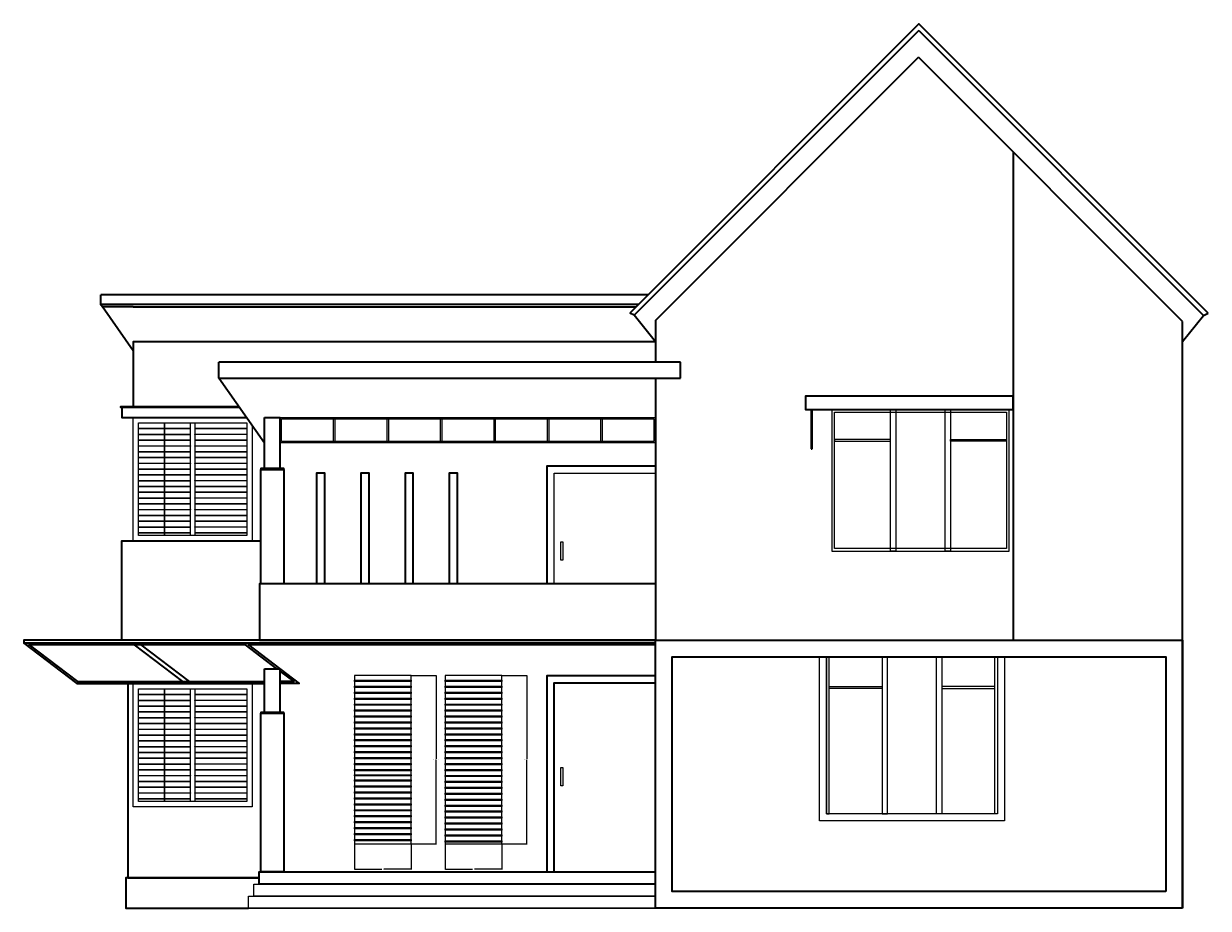
# Model space of a CAD drawing. Units: feet. Extents: x 2613 to 3913, y 950 to 1393.
# Tile 6 of 6: x 3319 to 3913, y 950 to 1393. Entities that reach past the tile are written whole.
import ezdxf

# ---------------------------------------------------------------- set-up
doc = ezdxf.new("R2010")
doc.units = ezdxf.units.FT
for name, color, linetype, lineweight in [('A-ANNO-DIMS', 2, 'Continuous', 18), ('A-DOOR', 3, 'Continuous', 25), ('A-ELEV', 7, 'Continuous', 35), ('A-FLOR-STRS', 7, 'Continuous', 25), ('A-GLAZ', 4, 'Continuous', 25), ('A-ROOF', 1, 'Continuous', 35)]:
    doc.layers.add(name, color=color, linetype=linetype, lineweight=lineweight)
doc.styles.get("Standard").update_dxf_attribs({"font": 'arial.ttf'})
doc.dimstyles.get("Standard").update_dxf_attribs({"dimtxt": 0.18, "dimasz": 0.18, "dimexe": 0.18, "dimexo": 0.0625, "dimgap": 0.09, "dimtad": 0, "dimtih": 1, "dimtoh": 1, "dimdec": 1, "dimzin": 0, "dimdsep": 46, "dimlunit": 3, "dimtxsty": 'Standard', "dimcen": 0.09, "dimadec": 0, "dimazin": 0, "dimtfac": 1, "dimtdec": 1, "dimtofl": 0, "dimtmove": 0, "dimatfit": 3, "dimfxl": 1, "dimtolj": 1, "dimtzin": 0, "dimarcsym": 0})

# ---------------------------------------------------------------- blocks, each defined once
blk = doc.blocks.new('WIN-LOUVRE-SHUTTER-L')
for points in [[(3513.53, 1066.37), (3485.15, 1066.37), (3485.15, 982.04), (3513.53, 982.04)], [(3485.15, 1064.05), (3513.53, 1064.05), (3513.53, 1063.39), (3485.15, 1063.39)], [(3485.15, 1061.07), (3513.53, 1061.07), (3513.53, 1060.41), (3485.15, 1060.41)], [(3485.15, 1058.09), (3513.53, 1058.09), (3513.53, 1057.43), (3485.15, 1057.43)], [(3485.15, 1055.11), (3513.53, 1055.11), (3513.53, 1054.45), (3485.15, 1054.45)], [(3485.15, 1052.13), (3513.53, 1052.13), (3513.53, 1051.47), (3485.15, 1051.47)], [(3485.15, 1049.15), (3513.53, 1049.15), (3513.53, 1048.49), (3485.15, 1048.49)], [(3485.15, 1046.18), (3513.53, 1046.18), (3513.53, 1045.51), (3485.15, 1045.51)], [(3485.15, 1043.2), (3513.53, 1043.2), (3513.53, 1042.53), (3485.15, 1042.53)], [(3485.15, 1040.22), (3513.53, 1040.22), (3513.53, 1039.56), (3485.15, 1039.56)], [(3485.15, 1037.24), (3513.53, 1037.24), (3513.53, 1036.58), (3485.15, 1036.58)], [(3485.15, 1034.26), (3513.53, 1034.26), (3513.53, 1033.6), (3485.15, 1033.6)], [(3485.15, 1031.28), (3513.53, 1031.28), (3513.53, 1030.62), (3485.15, 1030.62)], [(3485.15, 1028.3), (3513.53, 1028.3), (3513.53, 1027.64), (3485.15, 1027.64)], [(3485.15, 1025.32), (3513.53, 1025.32), (3513.53, 1024.66), (3485.15, 1024.66)], [(3485.15, 1022.34), (3513.53, 1022.34), (3513.53, 1021.68), (3485.15, 1021.68)], [(3485.15, 1019.36), (3513.53, 1019.36), (3513.53, 1018.7), (3485.15, 1018.7)], [(3485.15, 1016.71), (3513.53, 1016.71), (3513.53, 1016.05), (3485.15, 1016.05)], [(3485.15, 1014.07), (3513.53, 1014.07), (3513.53, 1013.4), (3485.15, 1013.4)], [(3485.15, 1011.09), (3513.53, 1011.09), (3513.53, 1010.43), (3485.15, 1010.43)], [(3485.15, 1008.11), (3513.53, 1008.11), (3513.53, 1007.45), (3485.15, 1007.45)], [(3485.15, 1005.13), (3513.53, 1005.13), (3513.53, 1004.47), (3485.15, 1004.47)], [(3485.15, 1002.15), (3513.53, 1002.15), (3513.53, 1001.49), (3485.15, 1001.49)], [(3485.15, 999.17), (3513.53, 999.17), (3513.53, 998.51), (3485.15, 998.51)], [(3485.15, 996.19), (3513.53, 996.19), (3513.53, 995.53), (3485.15, 995.53)], [(3485.15, 993.21), (3513.53, 993.21), (3513.53, 992.55), (3485.15, 992.55)], [(3485.15, 990.23), (3513.53, 990.23), (3513.53, 989.57), (3485.15, 989.57)], [(3485.15, 987.25), (3513.53, 987.25), (3513.53, 986.59), (3485.15, 986.59)], [(3485.15, 984.27), (3513.53, 984.27), (3513.53, 983.61), (3485.15, 983.61)]]:
    blk.add_lwpolyline(points, close=True)
blk = doc.blocks.new('WIN-LOUVRE-SHUTTER-R')
for points in [[(3559, 1066.37), (3530.62, 1066.37), (3530.62, 982.04), (3559, 982.04)], [(3530.62, 1064.05), (3559, 1064.05), (3559, 1063.39), (3530.62, 1063.39)], [(3530.62, 1061.07), (3559, 1061.07), (3559, 1060.41), (3530.62, 1060.41)], [(3530.62, 1058.09), (3559, 1058.09), (3559, 1057.43), (3530.62, 1057.43)], [(3530.62, 1055.11), (3559, 1055.11), (3559, 1054.45), (3530.62, 1054.45)], [(3530.62, 1052.13), (3559, 1052.13), (3559, 1051.47), (3530.62, 1051.47)], [(3530.62, 1049.15), (3559, 1049.15), (3559, 1048.49), (3530.62, 1048.49)], [(3530.62, 1046.18), (3559, 1046.18), (3559, 1045.51), (3530.62, 1045.51)], [(3530.62, 1043.2), (3559, 1043.2), (3559, 1042.53), (3530.62, 1042.53)], [(3530.62, 1040.22), (3559, 1040.22), (3559, 1039.56), (3530.62, 1039.56)], [(3530.62, 1037.24), (3559, 1037.24), (3559, 1036.58), (3530.62, 1036.58)], [(3530.62, 1034.26), (3559, 1034.26), (3559, 1033.6), (3530.62, 1033.6)], [(3530.62, 1031.28), (3559, 1031.28), (3559, 1030.62), (3530.62, 1030.62)], [(3530.62, 1028.3), (3559, 1028.3), (3559, 1027.64), (3530.62, 1027.64)], [(3530.62, 1025.32), (3559, 1025.32), (3559, 1024.66), (3530.62, 1024.66)], [(3530.62, 1022.34), (3559, 1022.34), (3559, 1021.68), (3530.62, 1021.68)], [(3530.62, 1019.36), (3559, 1019.36), (3559, 1018.7), (3530.62, 1018.7)], [(3530.62, 1016.38), (3559, 1016.38), (3559, 1015.72), (3530.62, 1015.72)], [(3530.62, 1013.4), (3559, 1013.4), (3559, 1012.74), (3530.62, 1012.74)], [(3530.62, 1010.43), (3559, 1010.43), (3559, 1009.76), (3530.62, 1009.76)], [(3530.62, 1007.45), (3559, 1007.45), (3559, 1006.78), (3530.62, 1006.78)], [(3530.62, 1004.47), (3559, 1004.47), (3559, 1003.81), (3530.62, 1003.81)], [(3530.62, 1001.49), (3559, 1001.49), (3559, 1000.83), (3530.62, 1000.83)], [(3530.62, 998.51), (3559, 998.51), (3559, 997.85), (3530.62, 997.85)], [(3530.62, 995.53), (3559, 995.53), (3559, 994.87), (3530.62, 994.87)], [(3530.62, 992.55), (3559, 992.55), (3559, 991.89), (3530.62, 991.89)], [(3530.62, 989.57), (3559, 989.57), (3559, 988.91), (3530.62, 988.91)], [(3530.62, 986.59), (3559, 986.59), (3559, 985.93), (3530.62, 985.93)], [(3530.62, 983.61), (3559, 983.61), (3559, 982.95), (3530.62, 982.95)]]:
    blk.add_lwpolyline(points, close=True)
blk = doc.blocks.new('*D3')
at = {"layer": 'A-ANNO-DIMS', "color": 0, "lineweight": -2, "transparency": 16777216}
for p, q in [((3513.59, 1066.37), (3526.36, 1066.37)), ((3526.18, 1066.19), (3526.18, 1024.41)), ((3526.18, 982.22), (3526.18, 1023.99)), ((3513.59, 982.04), (3526.36, 982.04))]:
    blk.add_line(p, q, dxfattribs=at)
at = {"layer": 'A-ANNO-DIMS', "color": 0, "transparency": 16777216}
for points in [[(3526.15, 1066.19), (3526.21, 1066.19), (3526.18, 1066.37)], [(3526.15, 982.22), (3526.21, 982.22), (3526.18, 982.04)]]:
    blk.add_solid(points, dxfattribs=at)
at = {"layer": 'Defpoints', "color": 0, "transparency": 16777216}
for p in [(3513.53, 1066.37), (3526.18, 1066.37), (3513.53, 982.04)]:
    blk.add_point(p, dxfattribs=at)
at = {"layer": 'A-ANNO-DIMS', "color": 0, "transparency": 16777216, "insert": (3526.18, 1024.2), "char_height": 0.18, "attachment_point": 5}
blk.add_mtext('\\A1;LOUVRE SHUTTER (L) 84 TYP.', dxfattribs=at)
blk = doc.blocks.new('*D4')
at = {"layer": 'A-ANNO-DIMS', "color": 0, "lineweight": -2, "transparency": 16777216}
for p, q in [((3485.15, 981.97), (3485.15, 969.21)), ((3513.53, 981.97), (3513.53, 969.21)), ((3485.33, 969.39), (3498.81, 969.39)), ((3513.35, 969.39), (3499.87, 969.39))]:
    blk.add_line(p, q, dxfattribs=at)
at = {"layer": 'A-ANNO-DIMS', "color": 0, "transparency": 16777216}
for points in [[(3485.33, 969.42), (3485.33, 969.36), (3485.15, 969.39)], [(3513.35, 969.42), (3513.35, 969.36), (3513.53, 969.39)]]:
    blk.add_solid(points, dxfattribs=at)
at = {"layer": 'Defpoints', "color": 0, "transparency": 16777216}
for p in [(3485.15, 982.04), (3513.53, 982.04), (3513.53, 969.39)]:
    blk.add_point(p, dxfattribs=at)
at = {"layer": 'A-ANNO-DIMS', "color": 0, "transparency": 16777216, "insert": (3499.34, 969.39), "char_height": 0.18, "attachment_point": 5}
blk.add_mtext('\\A1;28 TYP.', dxfattribs=at)
blk = doc.blocks.new('*D5')
at = {"layer": 'A-ANNO-DIMS', "color": 0, "lineweight": -2, "transparency": 16777216}
for p, q in [((3559.06, 1066.37), (3571.83, 1066.37)), ((3571.65, 1066.19), (3571.65, 1024.41)), ((3571.65, 982.22), (3571.65, 1023.99)), ((3559.06, 982.04), (3571.83, 982.04))]:
    blk.add_line(p, q, dxfattribs=at)
at = {"layer": 'A-ANNO-DIMS', "color": 0, "transparency": 16777216}
for points in [[(3571.62, 1066.19), (3571.68, 1066.19), (3571.65, 1066.37)], [(3571.62, 982.22), (3571.68, 982.22), (3571.65, 982.04)]]:
    blk.add_solid(points, dxfattribs=at)
at = {"layer": 'Defpoints', "color": 0, "transparency": 16777216}
for p in [(3559, 1066.37), (3571.65, 1066.37), (3559, 982.04)]:
    blk.add_point(p, dxfattribs=at)
at = {"layer": 'A-ANNO-DIMS', "color": 0, "transparency": 16777216, "insert": (3571.65, 1024.2), "char_height": 0.18, "attachment_point": 5}
blk.add_mtext('\\A1;LOUVRE SHUTTER (R) 84 TYP.', dxfattribs=at)
blk = doc.blocks.new('*D6')
at = {"layer": 'A-ANNO-DIMS', "color": 0, "lineweight": -2, "transparency": 16777216}
for p, q in [((3530.62, 981.97), (3530.62, 969.21)), ((3559, 981.97), (3559, 969.21)), ((3530.8, 969.39), (3544.28, 969.39)), ((3558.82, 969.39), (3545.34, 969.39))]:
    blk.add_line(p, q, dxfattribs=at)
at = {"layer": 'A-ANNO-DIMS', "color": 0, "transparency": 16777216}
for points in [[(3530.8, 969.42), (3530.8, 969.36), (3530.62, 969.39)], [(3558.82, 969.42), (3558.82, 969.36), (3559, 969.39)]]:
    blk.add_solid(points, dxfattribs=at)
at = {"layer": 'Defpoints', "color": 0, "transparency": 16777216}
for p in [(3530.62, 982.04), (3559, 982.04), (3559, 969.39)]:
    blk.add_point(p, dxfattribs=at)
at = {"layer": 'A-ANNO-DIMS', "color": 0, "transparency": 16777216, "insert": (3544.81, 969.39), "char_height": 0.18, "attachment_point": 5}
blk.add_mtext('\\A1;28 TYP.', dxfattribs=at)

msp = doc.modelspace()

# ---------------------------------------------------------------- linework, layer by layer
at = {"layer": 'A-DOOR'}
msp.add_lwpolyline([(3585.22, 1112.32), (3585.22, 1167.82), (3636.04, 1167.82), (3636.04, 1112.32)], dxfattribs=at)
for points in [[(3588.56, 1133.45), (3589.66, 1133.45), (3589.66, 1124.29), (3588.56, 1124.29)], [(3588.56, 1020.32), (3589.66, 1020.32), (3589.66, 1011.16), (3588.56, 1011.16)]]:
    msp.add_lwpolyline(points, close=True, dxfattribs=at)
at = {"layer": 'A-ELEV'}
for p, q in [((3374.19, 1229.14), (3358.75, 1251.12)), ((3636.04, 1233.69), (3625.42, 1247)), ((3900.4, 1233.84), (3910.94, 1246.9)), ((3900.4, 949.74), (3900.4, 1243.92)), ((3648.69, 1223.38), (3417.19, 1223.38)), ((3417.19, 1215.5), (3417.19, 1223.38)), ((3648.69, 1215.5), (3648.69, 1223.38)), ((3440.06, 1182.94), (3417.19, 1215.5)), ((3417.19, 1215.5), (3628.08, 1215.5)), ((3628.08, 1215.5), (3648.69, 1215.5)), ((3368.48, 1195.74), (3374.19, 1195.74)), ((3714.24, 1199.69), (3714.24, 1180.01)), ((3714.68, 1180.01), (3714.68, 1199.69)), ((3714.24, 1180.01), (3714.68, 1180.01)), ((3322.02, 1081.77), (3346.22, 1063.35)), ((3374.67, 1081.77), (3398.87, 1063.35)), ((3378.02, 1081.77), (3402.22, 1063.35)), ((3440.06, 1069.74), (3447.82, 1069.74)), ((3371.47, 1062.44), (3371.47, 965.01)), ((3371.47, 965.01), (3437.35, 964.93))]:
    msp.add_line(p, q, dxfattribs=at)
for points in [[(3815.51, 1328.81), (3815.51, 1084.12), (3900.4, 1084.12)], [(3636.04, 1244.29), (3636.04, 1223.38)], [(3900.4, 1084.12), (3900.4, 1243.92)], [(3636.04, 1233.69), (3374.19, 1233.69), (3374.19, 1229.14), (3374.19, 1201.16)], [(3636.04, 1215.5), (3636.04, 1084.12)], [(3427.6, 1200.68), (3368.08, 1200.68), (3368.08, 1201.16), (3427.27, 1201.16)], [(3427.6, 1200.68), (3368.48, 1200.68), (3368.48, 1195.74), (3431.07, 1195.74)], [(3581.76, 1112.32), (3581.76, 1171.49), (3636.04, 1171.49), (3636.04, 1112.32)], [(3438.29, 1112.32), (3438.29, 1169.74), (3449.67, 1169.74), (3449.67, 1112.32)], [(3470.3, 1112.32), (3470.3, 1167.82), (3466.17, 1167.82), (3466.17, 1112.32)], [(3492.47, 1112.32), (3492.47, 1167.82), (3488.34, 1167.82), (3488.34, 1112.32)], [(3514.64, 1112.32), (3514.64, 1167.82), (3510.51, 1167.82), (3510.51, 1112.32)], [(3536.82, 1112.32), (3536.82, 1167.82), (3532.69, 1167.82), (3532.69, 1112.32)], [(3437.59, 1091.48), (3437.59, 1084.12), (3368.48, 1084.12), (3368.48, 1133.88), (3438.29, 1133.88)], [(3636.04, 1112.32), (3437.59, 1112.32), (3437.59, 1084.12), (3636.04, 1084.12)], [(3636.04, 1082.68), (3319.31, 1082.68), (3345.91, 1062.44), (3440.06, 1062.44)], [(3446.31, 1069.74), (3430.51, 1081.77), (3322.02, 1081.77), (3346.22, 1063.35), (3440.06, 1063.35)], [(3636.04, 1081.77), (3432.02, 1081.77), (3457.42, 1062.44), (3447.82, 1062.44)], [(3447.82, 1068.59), (3454.7, 1063.35), (3447.82, 1063.35)], [(3581.76, 967.97), (3581.76, 1066.37), (3636.04, 1066.37)], [(3585.22, 967.97), (3585.22, 1062.69), (3636.04, 1062.69)], [(3437.35, 964.93), (3370.54, 964.93), (3370.54, 949.74), (3431.96, 949.74)], [(3636.04, 961.9), (3437.35, 961.9), (3437.35, 967.97), (3636.04, 967.97)]]:
    msp.add_lwpolyline(points, dxfattribs=at)
for points in [[(3815.51, 1206.47), (3711.34, 1206.47), (3711.34, 1199.69), (3815.51, 1199.69)], [(3440.06, 1195.74), (3447.82, 1195.74), (3447.82, 1170.13), (3440.06, 1170.13)], [(3438.21, 1169.74), (3449.67, 1169.74), (3449.67, 1170.13), (3438.21, 1170.13)], [(3319.31, 1082.68), (3636.04, 1082.68), (3636.04, 1084.12), (3319.31, 1084.12)], [(3900.4, 949.74), (3636.04, 949.74), (3636.04, 1084.12), (3900.4, 1084.12)], [(3892.05, 958.09), (3644.39, 958.09), (3644.39, 1075.78), (3892.05, 1075.78)], [(3440.06, 1069.74), (3447.82, 1069.74), (3447.82, 1047.95), (3440.06, 1047.95)], [(3438.21, 1047.56), (3449.67, 1047.56), (3449.67, 1047.95), (3438.21, 1047.95)], [(3438.29, 1047.56), (3449.67, 1047.56), (3449.67, 967.97), (3438.29, 967.97)]]:
    msp.add_lwpolyline(points, close=True, dxfattribs=at)
at = {"layer": 'A-FLOR-STRS'}
msp.add_line((3431.96, 949.74), (3900.4, 949.74), dxfattribs=at)
for points in [[(3636.04, 955.82), (3434.65, 955.82), (3434.65, 961.9), (3636.04, 961.9)], [(3636.04, 949.74), (3431.96, 949.74), (3431.96, 955.82), (3636.04, 955.82)]]:
    msp.add_lwpolyline(points, dxfattribs=at)
at = {"layer": 'A-GLAZ'}
for p, q in [((3376.89, 1193.04), (3402.91, 1193.04)), ((3376.89, 1059.73), (3402.91, 1059.73))]:
    msp.add_line(p, q, dxfattribs=at)
for points in [[(3433.87, 1191.76), (3433.87, 1133.88), (3374.19, 1133.88), (3374.19, 1195.74), (3431.07, 1195.74)], [(3807.58, 1075.78), (3807.58, 997.08), (3721.83, 997.08), (3721.83, 1075.78)]]:
    msp.add_lwpolyline(points, dxfattribs=at)
for points in [[(3447.82, 1195.74), (3636.04, 1195.74), (3636.04, 1183.04), (3447.82, 1183.04)], [(3448.55, 1195.09), (3635.31, 1195.09), (3635.31, 1183.7), (3448.55, 1183.7)], [(3474.7, 1195.09), (3475.36, 1195.09), (3475.36, 1183.7), (3474.7, 1183.7)], [(3501.51, 1195.09), (3502.17, 1195.09), (3502.17, 1183.7), (3501.51, 1183.7)], [(3528.32, 1195.09), (3528.97, 1195.09), (3528.97, 1183.7), (3528.32, 1183.7)], [(3555.13, 1195.09), (3555.78, 1195.09), (3555.78, 1183.7), (3555.13, 1183.7)], [(3581.93, 1195.09), (3582.59, 1195.09), (3582.59, 1183.7), (3581.93, 1183.7)], [(3608.74, 1195.09), (3609.4, 1195.09), (3609.4, 1183.7), (3608.74, 1183.7)], [(3813.46, 1199.69), (3724.51, 1199.69), (3724.51, 1128.72), (3813.46, 1128.72)], [(3725.89, 1198.4), (3812.08, 1198.4), (3812.08, 1130.01), (3725.89, 1130.01)], [(3753.94, 1199.69), (3756.61, 1199.69), (3756.61, 1128.72), (3753.94, 1128.72)], [(3781.29, 1199.69), (3783.97, 1199.69), (3783.97, 1128.72), (3781.29, 1128.72)], [(3376.89, 1193.04), (3431.17, 1193.04), (3431.17, 1136.58), (3376.89, 1136.58)], [(3376.89, 1190.17), (3402.91, 1190.17), (3402.91, 1190.14), (3376.89, 1190.14)], [(3389.88, 1193.04), (3389.91, 1193.04), (3389.91, 1136.58), (3389.88, 1136.58)], [(3402.91, 1193.04), (3405.15, 1193.04), (3405.15, 1136.58), (3402.91, 1136.58)], [(3405.15, 1190.21), (3431.17, 1190.21), (3431.17, 1190.14), (3405.15, 1190.14)], [(3376.89, 1187.27), (3402.91, 1187.27), (3402.91, 1187.24), (3376.89, 1187.24)], [(3376.89, 1184.37), (3402.91, 1184.37), (3402.91, 1184.34), (3376.89, 1184.34)], [(3405.15, 1187.31), (3431.17, 1187.31), (3431.17, 1187.24), (3405.15, 1187.24)], [(3405.15, 1184.4), (3431.17, 1184.4), (3431.17, 1184.34), (3405.15, 1184.34)], [(3753.94, 1184.76), (3725.89, 1184.76), (3725.89, 1183.78), (3753.94, 1183.78)], [(3783.97, 1184.76), (3812.08, 1184.76), (3812.08, 1183.78), (3783.97, 1183.78)], [(3376.89, 1181.47), (3402.91, 1181.47), (3402.91, 1181.44), (3376.89, 1181.44)], [(3376.89, 1178.57), (3402.91, 1178.57), (3402.91, 1178.53), (3376.89, 1178.53)], [(3405.15, 1181.5), (3431.17, 1181.5), (3431.17, 1181.44), (3405.15, 1181.44)], [(3405.15, 1178.6), (3431.17, 1178.6), (3431.17, 1178.53), (3405.15, 1178.53)], [(3376.89, 1175.67), (3402.91, 1175.67), (3402.91, 1175.63), (3376.89, 1175.63)], [(3376.89, 1172.76), (3402.91, 1172.76), (3402.91, 1172.73), (3376.89, 1172.73)], [(3405.15, 1175.7), (3431.17, 1175.7), (3431.17, 1175.63), (3405.15, 1175.63)], [(3405.15, 1172.8), (3431.17, 1172.8), (3431.17, 1172.73), (3405.15, 1172.73)], [(3376.89, 1169.86), (3402.91, 1169.86), (3402.91, 1169.83), (3376.89, 1169.83)], [(3376.89, 1166.96), (3402.91, 1166.96), (3402.91, 1166.93), (3376.89, 1166.93)], [(3405.15, 1169.9), (3431.17, 1169.9), (3431.17, 1169.83), (3405.15, 1169.83)], [(3405.15, 1166.99), (3431.17, 1166.99), (3431.17, 1166.93), (3405.15, 1166.93)], [(3376.89, 1164.06), (3402.91, 1164.06), (3402.91, 1164.03), (3376.89, 1164.03)], [(3376.89, 1161.16), (3402.91, 1161.16), (3402.91, 1161.12), (3376.89, 1161.12)], [(3405.15, 1164.09), (3431.17, 1164.09), (3431.17, 1164.03), (3405.15, 1164.03)], [(3405.15, 1161.19), (3431.17, 1161.19), (3431.17, 1161.12), (3405.15, 1161.12)], [(3405.15, 1158.29), (3431.17, 1158.29), (3431.17, 1158.22), (3405.15, 1158.22)], [(3376.89, 1158.25), (3402.91, 1158.25), (3402.91, 1158.22), (3376.89, 1158.22)], [(3376.89, 1155.35), (3402.91, 1155.35), (3402.91, 1155.32), (3376.89, 1155.32)], [(3376.89, 1152.45), (3402.91, 1152.45), (3402.91, 1152.42), (3376.89, 1152.42)], [(3405.15, 1155.39), (3431.17, 1155.39), (3431.17, 1155.32), (3405.15, 1155.32)], [(3405.15, 1152.48), (3431.17, 1152.48), (3431.17, 1152.42), (3405.15, 1152.42)], [(3376.89, 1149.55), (3402.91, 1149.55), (3402.91, 1149.52), (3376.89, 1149.52)], [(3376.89, 1146.65), (3402.91, 1146.65), (3402.91, 1146.61), (3376.89, 1146.61)], [(3405.15, 1149.58), (3431.17, 1149.58), (3431.17, 1149.52), (3405.15, 1149.52)], [(3405.15, 1146.68), (3431.17, 1146.68), (3431.17, 1146.61), (3405.15, 1146.61)], [(3376.89, 1143.75), (3402.91, 1143.75), (3402.91, 1143.71), (3376.89, 1143.71)], [(3376.89, 1140.84), (3402.91, 1140.84), (3402.91, 1140.81), (3376.89, 1140.81)], [(3405.15, 1143.78), (3431.17, 1143.78), (3431.17, 1143.71), (3405.15, 1143.71)], [(3405.15, 1140.88), (3431.17, 1140.88), (3431.17, 1140.81), (3405.15, 1140.81)], [(3376.89, 1137.94), (3402.91, 1137.94), (3402.91, 1137.91), (3376.89, 1137.91)], [(3405.15, 1137.98), (3431.17, 1137.98), (3431.17, 1137.91), (3405.15, 1137.91)], [(3718.35, 1075.78), (3811.06, 1075.78), (3811.06, 993.6), (3718.35, 993.6)], [(3723.17, 1075.78), (3721.83, 1075.78), (3721.83, 997.08), (3723.17, 997.08)], [(3752.36, 1075.78), (3749.69, 1075.78), (3749.69, 997.08), (3752.36, 997.08)], [(3777.05, 1075.78), (3779.72, 1075.78), (3779.72, 997.08), (3777.05, 997.08)], [(3806.24, 1075.78), (3807.58, 1075.78), (3807.58, 997.08), (3806.24, 997.08)], [(3374.19, 1062.44), (3433.87, 1062.44), (3433.87, 1000.58), (3374.19, 1000.58)], [(3376.89, 1059.73), (3431.17, 1059.73), (3431.17, 1003.28), (3376.89, 1003.28)], [(3389.88, 1059.73), (3389.91, 1059.73), (3389.91, 1003.28), (3389.88, 1003.28)], [(3402.91, 1059.73), (3405.15, 1059.73), (3405.15, 1003.28), (3402.91, 1003.28)], [(3723.17, 1060.85), (3749.69, 1060.85), (3749.69, 1059.87), (3723.17, 1059.87)], [(3806.24, 1060.85), (3779.72, 1060.85), (3779.72, 1059.87), (3806.24, 1059.87)], [(3376.89, 1056.87), (3402.91, 1056.87), (3402.91, 1056.83), (3376.89, 1056.83)], [(3376.89, 1053.96), (3402.91, 1053.96), (3402.91, 1053.93), (3376.89, 1053.93)], [(3405.15, 1056.9), (3431.17, 1056.9), (3431.17, 1056.83), (3405.15, 1056.83)], [(3405.15, 1054), (3431.17, 1054), (3431.17, 1053.93), (3405.15, 1053.93)], [(3376.89, 1051.06), (3402.91, 1051.06), (3402.91, 1051.03), (3376.89, 1051.03)], [(3376.89, 1048.16), (3402.91, 1048.16), (3402.91, 1048.13), (3376.89, 1048.13)], [(3405.15, 1051.1), (3431.17, 1051.1), (3431.17, 1051.03), (3405.15, 1051.03)], [(3405.15, 1048.19), (3431.17, 1048.19), (3431.17, 1048.13), (3405.15, 1048.13)], [(3376.89, 1045.26), (3402.91, 1045.26), (3402.91, 1045.23), (3376.89, 1045.23)], [(3376.89, 1042.36), (3402.91, 1042.36), (3402.91, 1042.32), (3376.89, 1042.32)], [(3405.15, 1045.29), (3431.17, 1045.29), (3431.17, 1045.23), (3405.15, 1045.23)], [(3405.15, 1042.39), (3431.17, 1042.39), (3431.17, 1042.32), (3405.15, 1042.32)], [(3405.15, 1039.49), (3431.17, 1039.49), (3431.17, 1039.42), (3405.15, 1039.42)], [(3376.89, 1039.46), (3402.91, 1039.46), (3402.91, 1039.42), (3376.89, 1039.42)], [(3376.89, 1036.55), (3402.91, 1036.55), (3402.91, 1036.52), (3376.89, 1036.52)], [(3376.89, 1033.65), (3402.91, 1033.65), (3402.91, 1033.62), (3376.89, 1033.62)], [(3405.15, 1036.59), (3431.17, 1036.59), (3431.17, 1036.52), (3405.15, 1036.52)], [(3405.15, 1033.69), (3431.17, 1033.69), (3431.17, 1033.62), (3405.15, 1033.62)], [(3376.89, 1030.75), (3402.91, 1030.75), (3402.91, 1030.72), (3376.89, 1030.72)], [(3376.89, 1027.85), (3402.91, 1027.85), (3402.91, 1027.82), (3376.89, 1027.82)], [(3405.15, 1030.78), (3431.17, 1030.78), (3431.17, 1030.72), (3405.15, 1030.72)], [(3405.15, 1027.88), (3431.17, 1027.88), (3431.17, 1027.82), (3405.15, 1027.82)], [(3376.89, 1024.95), (3402.91, 1024.95), (3402.91, 1024.91), (3376.89, 1024.91)], [(3376.89, 1022.05), (3402.91, 1022.05), (3402.91, 1022.01), (3376.89, 1022.01)], [(3405.15, 1024.98), (3431.17, 1024.98), (3431.17, 1024.91), (3405.15, 1024.91)], [(3405.15, 1022.08), (3431.17, 1022.08), (3431.17, 1022.01), (3405.15, 1022.01)], [(3376.89, 1019.14), (3402.91, 1019.14), (3402.91, 1019.11), (3376.89, 1019.11)], [(3376.89, 1016.24), (3402.91, 1016.24), (3402.91, 1016.21), (3376.89, 1016.21)], [(3405.15, 1019.18), (3431.17, 1019.18), (3431.17, 1019.11), (3405.15, 1019.11)], [(3405.15, 1016.28), (3431.17, 1016.28), (3431.17, 1016.21), (3405.15, 1016.21)], [(3376.89, 1013.34), (3402.91, 1013.34), (3402.91, 1013.31), (3376.89, 1013.31)], [(3376.89, 1010.44), (3402.91, 1010.44), (3402.91, 1010.41), (3376.89, 1010.41)], [(3405.15, 1013.37), (3431.17, 1013.37), (3431.17, 1013.31), (3405.15, 1013.31)], [(3405.15, 1010.47), (3431.17, 1010.47), (3431.17, 1010.41), (3405.15, 1010.41)], [(3376.89, 1007.54), (3402.91, 1007.54), (3402.91, 1007.5), (3376.89, 1007.5)], [(3376.89, 1004.64), (3402.91, 1004.64), (3402.91, 1004.6), (3376.89, 1004.6)], [(3405.15, 1007.57), (3431.17, 1007.57), (3431.17, 1007.5), (3405.15, 1007.5)], [(3405.15, 1004.67), (3431.17, 1004.67), (3431.17, 1004.6), (3405.15, 1004.6)]]:
    msp.add_lwpolyline(points, close=True, dxfattribs=at)
at = {"layer": 'A-ROOF'}
for p, q in [((3768.13, 1389.71), (3625.42, 1247)), ((3768.13, 1389.71), (3910.94, 1246.9)), ((3636.04, 1244.29), (3768.03, 1376.28)), ((3900.4, 1243.92), (3768.03, 1376.28)), ((3374.19, 1257.12), (3357.93, 1257.12)), ((3357.93, 1252.28), (3357.93, 1257.12)), ((3632.25, 1257.12), (3374.19, 1257.12)), ((3627.41, 1252.28), (3357.93, 1252.28)), ((3374.19, 1251.12), (3358.75, 1251.12)), ((3374.19, 1251.12), (3626.25, 1251.12)), ((3625.42, 1247), (3623.19, 1248.06)), ((3910.94, 1246.9), (3913.29, 1248.02))]:
    msp.add_line(p, q, dxfattribs=at)
msp.add_lwpolyline([(3913.29, 1248.02), (3768.22, 1393.09), (3623.19, 1248.06)], dxfattribs=at)
msp.add_arc((3356.36, 1250.31), 2.52, 18.64427, 51.52327, dxfattribs=at)

# ---------------------------------------------------------------- block references
at = {"layer": 'A-GLAZ'}
for name in ['WIN-LOUVRE-SHUTTER-L', 'WIN-LOUVRE-SHUTTER-R']:
    msp.add_blockref(name, (0, 0), dxfattribs=at)

# ---------------------------------------------------------------- dimensions: what is measured, and where the dimension line sits
at = {"layer": 'A-ANNO-DIMS'}
for base, p1, p2, text, picture, middle in [((3526.18, 1066.37), (3513.53, 982.04), (3513.53, 1066.37), 'LOUVRE SHUTTER (L) <> TYP.', '*D3', (3526.18, 1024.2)), ((3571.65, 1066.37), (3559, 982.04), (3559, 1066.37), 'LOUVRE SHUTTER (R) <> TYP.', '*D5', (3571.65, 1024.2))]:
    dim = msp.add_linear_dim(base=base, p1=p1, p2=p2, angle=90, text=text, dimstyle='Standard', override={"dimdec": 0, "dimlfac": 1, "dimrnd": 0, "dimzin": 0, "dimdsep": 46, "dimlunit": 2}, dxfattribs=at)
    dim.commit()
    dim.dimension.update_dxf_attribs({"geometry": picture, "text_midpoint": middle})
for base, p1, p2, picture, middle in [((3513.53, 969.39), (3485.15, 982.04), (3513.53, 982.04), '*D4', (3499.34, 969.39)), ((3559, 969.39), (3530.62, 982.04), (3559, 982.04), '*D6', (3544.81, 969.39))]:
    dim = msp.add_linear_dim(base=base, p1=p1, p2=p2, text='<> TYP.', dimstyle='Standard', override={"dimdec": 0, "dimlfac": 1, "dimrnd": 0, "dimzin": 0, "dimdsep": 46, "dimlunit": 2}, dxfattribs=at)
    dim.commit()
    dim.dimension.update_dxf_attribs({"geometry": picture, "text_midpoint": middle})

doc.saveas('drawing.dxf')
